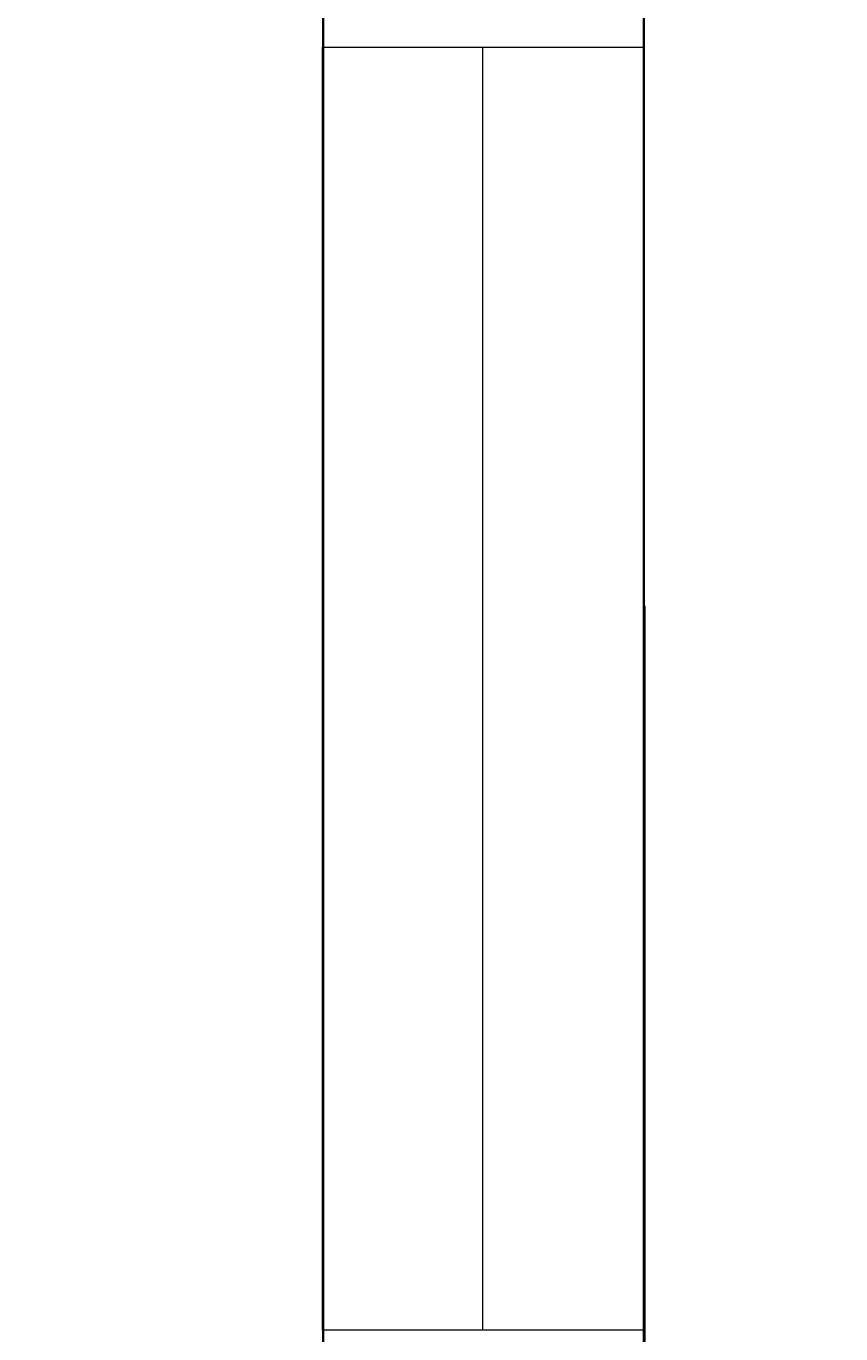
# Model space of a CAD drawing. Units: millimetres. Extents: x 27017497 to 27018854, y 7058029 to 7059154.
# Tile 15 of 91: x 27017605 to 27017628, y 7058238 to 7058275. Entities that reach past the tile are written whole.
import ezdxf

# ---------------------------------------------------------------- set-up
doc = ezdxf.new("R2010")
doc.units = ezdxf.units.MM
for name, color, linetype, lineweight in [('A-ANNO-DIMS', 2, 'Continuous', 18), ('A-FLOR-CASE', 8, 'Continuous', 20), ('A-GLAZ', 4, 'Continuous', 18), ('A-WALL', 7, 'Continuous', 35)]:
    doc.layers.add(name, color=color, linetype=linetype, lineweight=lineweight)
doc.styles.get("Standard").update_dxf_attribs({"font": 'arial.ttf'})
doc.dimstyles.get("Standard").update_dxf_attribs({"dimtxt": 0.18, "dimasz": 0.18, "dimexe": 0.18, "dimexo": 0.0625, "dimgap": 0.09, "dimtad": 0, "dimtih": 1, "dimtoh": 1, "dimdec": 4, "dimzin": 0, "dimdsep": 46, "dimtxsty": 'Standard', "dimcen": 0.09, "dimadec": 0, "dimazin": 0, "dimtfac": 1, "dimtdec": 4, "dimtofl": 0, "dimtmove": 0, "dimatfit": 3, "dimfxl": 1, "dimtolj": 1, "dimtzin": 0, "dimarcsym": 0})

# ---------------------------------------------------------------- blocks, each defined once
blk = doc.blocks.new('WINDOW-SINGLE-LIGHT')
blk.add_lwpolyline([(36, 4.5), (36, 0), (0, 0), (0, 9), (36, 9), (36, 4.5), (0, 4.5)])
blk = doc.blocks.new('*D47')
at = {"layer": 'A-ANNO-DIMS', "color": 0, "lineweight": -2, "transparency": 16777216}
for p, q in [((27017561.166, 7058294.35), (27017561.166, 7058028.6)), ((27018790.606, 7058294.35), (27018790.606, 7058028.6)), ((27017561.346, 7058028.78), (27018175.431, 7058028.78)), ((27018790.426, 7058028.78), (27018176.341, 7058028.78))]:
    blk.add_line(p, q, dxfattribs=at)
at = {"layer": 'A-ANNO-DIMS', "color": 0, "transparency": 16777216}
for points in [[(27017561.346, 7058028.81), (27017561.346, 7058028.75), (27017561.166, 7058028.78)], [(27018790.426, 7058028.81), (27018790.426, 7058028.75), (27018790.606, 7058028.78)]]:
    blk.add_solid(points, dxfattribs=at)
at = {"layer": 'Defpoints', "color": 0, "transparency": 16777216}
for p in [(27017561.166, 7058294.412), (27018790.606, 7058294.412), (27018790.606, 7058028.78)]:
    blk.add_point(p, dxfattribs=at)
at = {"layer": 'A-ANNO-DIMS', "color": 0, "transparency": 16777216, "insert": (27018175.886, 7058028.78), "char_height": 0.18, "attachment_point": 5}
blk.add_mtext('\\A1;1229.4', dxfattribs=at)
blk = doc.blocks.new('*D48')
at = {"layer": 'A-ANNO-DIMS', "color": 0, "lineweight": -2, "transparency": 16777216}
for p, q in [((27018463.498, 7058622.912), (27017497.536, 7058622.912)), ((27017497.716, 7058622.732), (27017497.716, 7058357.753)), ((27017497.716, 7058092.41), (27017497.716, 7058357.389)), ((27018555.129, 7058092.23), (27017497.536, 7058092.23))]:
    blk.add_line(p, q, dxfattribs=at)
at = {"layer": 'A-ANNO-DIMS', "color": 0, "transparency": 16777216}
for points in [[(27017497.686, 7058622.732), (27017497.746, 7058622.732), (27017497.716, 7058622.912)], [(27017497.686, 7058092.41), (27017497.746, 7058092.41), (27017497.716, 7058092.23)]]:
    blk.add_solid(points, dxfattribs=at)
at = {"layer": 'Defpoints', "color": 0, "transparency": 16777216}
for p in [(27018463.561, 7058622.912), (27017497.716, 7058092.23), (27018555.192, 7058092.23)]:
    blk.add_point(p, dxfattribs=at)
at = {"layer": 'A-ANNO-DIMS', "color": 0, "transparency": 16777216, "insert": (27017497.716, 7058357.571), "char_height": 0.18, "attachment_point": 5}
blk.add_mtext('\\A1;530.7', dxfattribs=at)

msp = doc.modelspace()

# ---------------------------------------------------------------- linework, layer by layer
at = {"layer": 'A-FLOR-CASE'}
msp.add_line((27017622.691, 7058258.237), (27017622.691, 7058207.055), dxfattribs=at)
at = {"layer": 'A-WALL'}
for p, q in [((27017613.666, 7058294.412), (27017613.666, 7058132.912)), ((27017622.666, 7058294.412), (27017622.666, 7058141.912))]:
    msp.add_line(p, q, dxfattribs=at)

# ---------------------------------------------------------------- block references
at = {"layer": 'A-GLAZ', "rotation": 270}
msp.add_blockref('WINDOW-SINGLE-LIGHT', (27017613.647, 7058273.913), dxfattribs=at)

# ---------------------------------------------------------------- dimensions: what is measured, and where the dimension line sits
at = {"layer": 'A-ANNO-DIMS'}
dim = msp.add_linear_dim(base=(27017497.716, 7058092.23), p1=(27018463.561, 7058622.912), p2=(27018555.192, 7058092.23), angle=90, dimstyle='Standard', override={"dimdec": 1, "dimlfac": 1, "dimrnd": 0, "dimzin": 0, "dimdsep": 46, "dimlunit": 2}, dxfattribs=at)
dim.commit()
dim.dimension.update_dxf_attribs({"geometry": '*D48', "text_midpoint": (27017497.716, 7058357.571)})
dim = msp.add_linear_dim(base=(27018790.606, 7058028.78), p1=(27017561.166, 7058294.412), p2=(27018790.606, 7058294.412), dimstyle='Standard', override={"dimdec": 1, "dimlfac": 1, "dimrnd": 0, "dimzin": 0, "dimdsep": 46, "dimlunit": 2}, dxfattribs=at)
dim.commit()
dim.dimension.update_dxf_attribs({"geometry": '*D47', "text_midpoint": (27018175.886, 7058028.78)})

doc.saveas('drawing.dxf')
